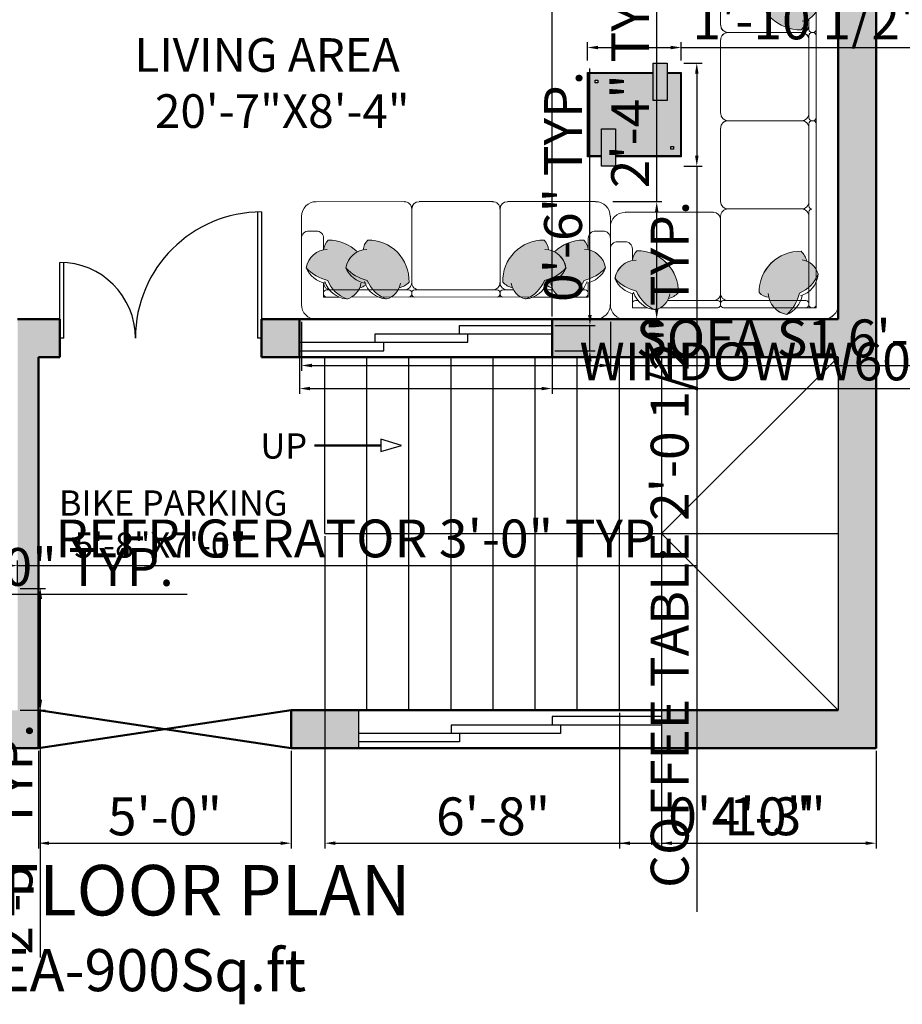
# Model space of a CAD drawing. Units: inches. Extents: x 3274 to 5176, y 1085 to 2172.
# Tile 7 of 16: x 3530 to 3740, y 1614 to 1848. Entities that reach past the tile are written whole.
import ezdxf

# ---------------------------------------------------------------- set-up
doc = ezdxf.new("R2010")
doc.units = ezdxf.units.IN
for name, color, linetype, lineweight in [('A-ANNO-DIMS', 2, 'Continuous', 18), ('A-ANNO-TEXT', 7, 'Continuous', 25), ('A-AREA-IDEN', 3, 'Continuous', 25), ('A-DOOR', 4, 'Continuous', 25), ('A-FLOR-FIXT', 8, 'Continuous', 18), ('A-FLOR-STRS', 7, 'Continuous', 25), ('A-FURN', 8, 'Continuous', 18), ('A-GLAZ', 5, 'Continuous', 25), ('A-WALL', 7, 'Continuous', 50), ('A-WALL-PATT', 8, 'Continuous', 13)]:
    doc.layers.add(name, color=color, linetype=linetype, lineweight=lineweight)
doc.layers.add('MOBIL', color=7, linetype='Continuous')
doc.styles.get("Standard").update_dxf_attribs({"font": 'arial.ttf'})
doc.dimstyles.new('ISO-25', dxfattribs={"dimtxt": 9, "dimasz": 2.5, "dimexe": 1.25, "dimexo": 0.625, "dimtad": 1, "dimdec": 1, "dimlunit": 3, "dimtxsty": 'Standard', "dimcen": 2.5, "dimclrd": 4, "dimclre": 4, "dimclrt": 1, "dimadec": 0, "dimazin": 0, "dimtfac": 1, "dimtdec": 1, "dimtmove": 0, "dimatfit": 3, "dimfxl": 1, "dimarcsym": 0})

# ---------------------------------------------------------------- blocks, each defined once
blk = doc.blocks.new('3')
for p, q in [((47, 30), (47, 0)), ((48, 30), (48, 0)), ((0, 0), (0, 18)), ((1, 0), (1, 18)), ((1, 0), (0, 0)), ((48, 0), (47, 0))]:
    blk.add_line(p, q)
for centre, radius, start, end in [((48, 0), 30, 90, 180), ((0, 0), 18, 0, 90)]:
    blk.add_arc(centre, radius, start, end)
blk = doc.blocks.new('SOFA 1')
at = {"transparency": 33554687}
h = blk.add_hatch(color=256, dxfattribs=at)
h.dxf.hatch_style = 1
h.paths.add_polyline_path([(3723.52, 1308.63, 0.147724), (3717.76, 1305.24, 0.310469), (3722.42, 1300.4), (3722.42, 1300.25, 0.156703), (3723.62, 1297.8, 0.425821), (3734.69, 1309.08, 0.121928), (3732.05, 1310.63, 0.233216), (3728.6, 1313.59, 0.213835)])
h = blk.add_hatch(color=256, dxfattribs=at)
h.dxf.hatch_style = 1
h.paths.add_polyline_path([(3769.65, 1307.6, 0.084911), (3767.15, 1309.12, 0.046133), (3766.46, 1311.13), (3759.18, 1311.13, 0.039409), (3758.92, 1310.24, 0.165523), (3756.31, 1309.02, 0.42585), (3767.59, 1297.95, 0.121928), (3769.15, 1300.58, 0.027403), (3769.65, 1300.83)])
h.paths.add_polyline_path([(3765.34, 1313.08), (3760.4, 1313.08, 0.097704), (3759.18, 1311.13), (3766.46, 1311.13, 0.04873)])
h.paths.add_polyline_path([(3763.76, 1314.88, 0.16488), (3760.4, 1313.08), (3765.34, 1313.08, 0.051917)])
h.paths.add_polyline_path([(3771.6, 1305.17, 0.090388), (3769.65, 1307.6), (3769.65, 1300.83, 0.136035), (3771.6, 1302.77)])
h = blk.add_hatch(color=256, dxfattribs=at)
h.dxf.hatch_style = 1
h.paths.add_polyline_path([(3769.16, 1235.96, 0.122267), (3767.6, 1238.61, 0.425972), (3756.32, 1227.54, 0.165563), (3758.93, 1226.32, 0.309481), (3763.76, 1221.69, 0.002677), (3763.83, 1221.72, 0.146094), (3767.16, 1227.43, 0.212433), (3772.1, 1232.48, 0.235342)])
h = blk.add_hatch(color=256, dxfattribs=at)
h.dxf.hatch_style = 1
h.paths.add_polyline_path([(3769.16, 1225.36, 0.122267), (3767.6, 1228.01, 0.425972), (3756.32, 1216.94, 0.165563), (3758.93, 1215.72, 0.309481), (3763.76, 1211.09, 0.002677), (3763.83, 1211.12, 0.146094), (3767.16, 1216.83, 0.212433), (3772.1, 1221.88, 0.235342)])
for p, q in [((3720.45, 1316.13), (3773.58, 1316.13)), ((3777.51, 1312.19), (3777.51, 1213.72))]:
    blk.add_line(p, q, dxfattribs=at)
for points in [[(3717.76, 1305.24, -0.147724), (3723.52, 1308.63, -0.213355), (3728.59, 1313.59, 0.213355), (3723.52, 1308.63, 0.147724), (3717.76, 1305.24, -0.249545), (3722.86, 1309.34, 0.249545), (3717.75, 1305.25, 0.356779), (3723.4, 1300.28, -0.356779), (3717.76, 1305.24)], [(3728.58, 1313.6, -0.306333), (3732.42, 1309.31, 0.306333), (3728.58, 1313.6, 0.306674), (3722.72, 1308.89, -0.306674), (3728.58, 1313.6)], [(3763.76, 1314.88, -0.147724), (3767.15, 1309.12, -0.213355), (3772.1, 1304.05, 0.213355), (3767.15, 1309.12, 0.147724), (3763.76, 1314.88, -0.249545), (3767.86, 1309.77, 0.249545), (3763.77, 1314.89, 0.356779), (3758.8, 1309.23, -0.356779), (3763.76, 1314.88)], [(3734.69, 1309.08, -0.425972), (3723.62, 1297.8, -0.165552), (3722.4, 1300.4, 0.165552), (3723.62, 1297.79, 0.425972), (3734.69, 1309.07, 0.121514), (3732.07, 1310.63, -0.121514), (3734.69, 1309.08)], [(3767.6, 1297.95, -0.425972), (3756.31, 1309.01, -0.165552), (3758.92, 1310.24, 0.165552), (3756.31, 1309.02, 0.425972), (3767.59, 1297.95, 0.121514), (3769.14, 1300.57, -0.121514), (3767.6, 1297.95)], [(3772.11, 1304.06, -0.306333), (3767.83, 1300.22, 0.306333), (3772.11, 1304.06, 0.306674), (3767.4, 1309.91, -0.306674), (3772.11, 1304.06)], [(3770.44, 1286.63, -0.414214), (3769.66, 1287.4, 0.414214), (3770.44, 1286.63, 0.414214), (3769.66, 1285.83, -0.414214), (3770.44, 1286.63)], [(3748.01, 1262.99, -0.414214), (3746.05, 1264.95, 0.414214), (3748.01, 1262.97, 0.414213), (3746.05, 1261.01, -0.414213), (3748.01, 1262.99)], [(3770.44, 1262.99, -0.414214), (3769.66, 1263.77, 0.414214), (3770.44, 1262.99, 0.414214), (3769.66, 1262.19, -0.414214), (3770.44, 1262.99)], [(3770.83, 1262.97, -0.414214), (3771.61, 1262.19, 0.414214), (3770.83, 1262.99, 0.414214), (3771.61, 1263.77, -0.414214), (3770.83, 1262.97)], [(3748.01, 1239.35, -0.414214), (3746.05, 1241.31, 0.414214), (3748.01, 1239.33, 0.414213), (3746.05, 1237.37, -0.414213), (3748.01, 1239.35)], [(3767.7, 1239.33, -0.414214), (3769.66, 1237.37, 0.414214), (3767.7, 1239.35, 0.414214), (3769.66, 1241.31, -0.414214), (3767.7, 1239.33)], [(3770.44, 1239.35, -0.414214), (3769.66, 1240.13, 0.414214), (3770.44, 1239.33, 0.414214), (3769.66, 1238.55, -0.414214), (3770.44, 1239.35)], [(3770.83, 1239.33, -0.414214), (3771.61, 1238.55, 0.414214), (3770.83, 1239.35, 0.414214), (3771.61, 1240.13, -0.414214), (3770.83, 1239.33)], [(3756.32, 1227.54, -0.425972), (3767.6, 1238.61, -0.121514), (3769.16, 1235.98, 0.121514), (3767.6, 1238.61, 0.425972), (3756.32, 1227.54, 0.165552), (3758.93, 1226.32, -0.165552), (3756.32, 1227.54)], [(3772.1, 1232.5, -0.306674), (3767.41, 1226.64, 0.306674), (3772.1, 1232.5, 0.306333), (3767.84, 1236.34, -0.306333), (3772.1, 1232.5)], [(3763.78, 1221.67, 0.249545), (3767.87, 1226.78, -0.249545), (3763.76, 1221.69, -0.356779), (3758.81, 1227.32, 0.356779), (3763.77, 1221.68, 0.147724), (3767.16, 1227.43, 0.213355), (3772.11, 1232.51, -0.213355), (3767.16, 1227.43, -0.147724), (3763.78, 1221.67)], [(3756.32, 1216.94, -0.200233), (3759.49, 1224.76, 0.200233), (3756.32, 1216.94, 0.165552), (3758.93, 1215.72, -0.165552), (3756.32, 1216.94)], [(3772.1, 1221.9, -0.306674), (3767.41, 1216.04, 0.306674), (3772.1, 1221.9, -0.213355), (3767.16, 1216.83, -0.147724), (3763.77, 1211.08, 0.147724), (3767.15, 1216.83, 0.213355), (3772.1, 1221.9)], [(3763.76, 1211.09, -0.356779), (3758.81, 1216.72, 0.356779), (3763.76, 1211.09, 0.249545), (3767.87, 1216.18, -0.249545), (3763.76, 1211.09)]]:
    blk.add_lwpolyline(points, format="xyb", dxfattribs=at)
for points in [[(3716.51, 1312.2), (3716.51, 1291.44)], [(3722.42, 1313.08), (3722.42, 1309.23), (3722.42, 1313.08), (3726.57, 1313.08)], [(3723.21, 1311.13), (3723.93, 1311.13)], [(3729.85, 1313.08), (3745.25, 1313.08)], [(3731.82, 1311.13), (3745.25, 1311.13)], [(3746.01, 1312.3), (3746.01, 1288.55)], [(3746.01, 1310.97), (3746.01, 1311.36)], [(3768.11, 1313.08), (3746.78, 1313.08)], [(3768.87, 1311.13), (3746.78, 1311.13)], [(3771.6, 1313.08), (3767.75, 1313.08), (3771.6, 1313.08), (3771.6, 1308.93)], [(3769.66, 1287.39), (3769.65, 1312.3)], [(3771.6, 1313.08), (3771.61, 1233.74)], [(3746.01, 1288.54), (3746.01, 1308.23)], [(3769.65, 1309.43), (3769.65, 1308.71)], [(3722.42, 1300.39), (3722.42, 1297.33)], [(3720.45, 1295.38), (3718.48, 1295.38)], [(3720.45, 1287.5), (3744.09, 1287.5)], [(3746.02, 1284.63), (3746.02, 1264.94)], [(3747.99, 1286.6), (3767.69, 1286.6)], [(3769.66, 1263.75), (3769.66, 1285.81)], [(3769.66, 1277.18), (3769.66, 1263.75)], [(3746.02, 1260.99), (3746.02, 1241.3)], [(3747.99, 1262.97), (3767.69, 1262.97)], [(3769.66, 1240.12), (3769.66, 1262.18)], [(3770.43, 1262.97), (3770.82, 1262.97)], [(3746.02, 1237.36), (3746.02, 1213.74)], [(3747.99, 1239.33), (3767.69, 1239.33)], [(3769.66, 1235.71), (3769.66, 1238.54)], [(3770.43, 1239.33), (3770.82, 1239.33)], [(3771.61, 1223.14), (3771.61, 1230.47)], [(3769.66, 1225.11), (3769.66, 1227.82)], [(3767.76, 1215.72), (3771.61, 1215.72), (3771.61, 1219.84), (3771.61, 1215.72)], [(3769.66, 1216.5), (3769.66, 1217.22)], [(3753.91, 1211.77), (3753.91, 1213.74)], [(3755.86, 1215.72), (3758.92, 1215.72)], [(3749.97, 1209.8), (3773.58, 1209.8)]]:
    blk.add_lwpolyline(points, close=True, dxfattribs=at)
for points in [[(3722.42, 1311.91, 0.414214), (3723.2, 1311.13, -0.414214)], [(3770.43, 1313.08, 0.414214), (3769.65, 1312.3, -0.414214)], [(3771.6, 1312.3, 0.414214), (3770.82, 1313.08, -0.414214)], [(3716.51, 1297.34, 0.414214), (3718.47, 1295.38, -0.414214)], [(3720.44, 1295.38, 0.414214), (3722.4, 1297.34, -0.414214)], [(3716.51, 1291.45, 0.414212), (3720.44, 1287.52, -0.414212)], [(3746.03, 1288.56, 0.414214), (3747.99, 1286.6, 0.414213), (3746.03, 1284.64, -0.414213), (3747.99, 1286.6, -0.414214)], [(3769.66, 1284.64, 0.414214), (3767.7, 1286.6, 0.414214), (3769.66, 1288.56, -0.414214), (3767.7, 1286.6, -0.414214)], [(3769.66, 1261.01, 0.414214), (3767.7, 1262.97, 0.414214), (3769.66, 1264.93, -0.414214), (3767.7, 1262.97, -0.414214)], [(3769.16, 1225.36, 0.071861), (3768.39, 1227.01, -0.071861)], [(3772.13, 1221.9, 0.306333), (3767.84, 1225.74, -0.306333)], [(3769.66, 1216.52, 0.414214), (3770.44, 1215.74, -0.414214)], [(3770.83, 1215.74, 0.414214), (3771.61, 1216.52, -0.414214)], [(3746.05, 1213.76, 0.414212), (3749.98, 1209.82, -0.414212)], [(3755.87, 1215.72, 0.414214), (3753.91, 1213.76, -0.414214)], [(3755.87, 1209.8, -0.414214), (3753.91, 1211.76, 0.414214)]]:
    blk.add_lwpolyline(points, format="xyb", close=True, dxfattribs=at)
for centre, radius, start, end in [((3720.44, 1312.2), 3.93, 90.0002, 179.9998), ((3720.44, 1312.19), 3.94, 89.9158, 179.9154), ((3773.58, 1312.2), 3.93, 0.0002, 89.9998), ((3773.57, 1312.19), 3.94, 359.9158, 89.9154), ((3744.09, 1309.21), 1.92, 358.766, 90.5111), ((3745.22, 1312.29), 0.789, 0.8425, 90.8425), ((3745.24, 1311.91), 0.777, 270, 0), ((3745.24, 1311.91), 0.777, 270, 0), ((3746.8, 1312.29), 0.789, 89.1575, 179.1575), ((3746.79, 1311.91), 0.777, 180, 270), ((3746.79, 1311.91), 0.777, 180, 270), ((3747.93, 1309.21), 1.92, 89.4889, 181.234), ((3768.87, 1312.3), 0.777, 360, 90), ((3768.87, 1311.91), 0.777, 270, 0), ((3744.08, 1289.48), 1.96, 270, 360), ((3744.08, 1289.48), 1.96, 270, 360), ((3773.58, 1213.73), 3.93, 270.0002, 359.9998), ((3773.59, 1213.73), 3.93, 269.9156, 359.9152)]:
    blk.add_arc(centre, radius, start, end, dxfattribs=at)
blk = doc.blocks.new('Mesa de centro Cantria feeling')
at = {"layer": 'MOBIL', "ltscale": 0.2}
h = blk.add_hatch(color=256, dxfattribs=at)
h.set_gradient(color1=(74, 55, 38), color2=(104, 77, 54), one_color=1, tint=0.31, name='CYLINDER')
h.paths.add_polyline_path([(-0.85, -0.3), (-0.7, -0.3), (-0.7, 0.1), (-0.85, 0.1)])
h = blk.add_hatch(color=256, dxfattribs=at)
h.set_gradient(color1=(221, 221, 223), one_color=1, tint=1)
h.paths.add_polyline_path([(-0.15, -0.6), (-0.15, -0.89), (-0.01, -0.89), (-0.01, -0.01), (-0.7, -0.01), (-0.7, -0.3), (-0.85, -0.3), (-0.85, -0.01), (-0.99, -0.01), (-0.99, -0.89), (-0.3, -0.89), (-0.3, -0.6)])
h.paths.add_polyline_path([(-0.112, -0.112), (-0.112, -0.082), (-0.082, -0.082), (-0.082, -0.112)], flags=16)
h.paths.add_polyline_path([(-0.888, -0.788), (-0.888, -0.818), (-0.918, -0.818), (-0.918, -0.788)], flags=16)
h = blk.add_hatch(color=256, dxfattribs=at)
h.set_gradient(color1=(74, 55, 38), color2=(104, 77, 54), one_color=1, tint=0.31, name='CYLINDER')
h.paths.add_polyline_path([(-0.15, -0.6), (-0.3, -0.6), (-0.3, -1), (-0.15, -1)])
for points in [[(-0.85, 0), (-1, 0), (-1, -0.9), (-0.3, -0.9)], [(-0.15, -0.9), (0, -0.9), (0, 0), (-0.7, 0)], [(-0.85, -0.01), (-0.99, -0.01), (-0.99, -0.89), (-0.3, -0.89)], [(-0.15, -0.89), (-0.01, -0.89), (-0.01, -0.01), (-0.7, -0.01)]]:
    blk.add_lwpolyline(points, dxfattribs=at)
for points in [[(-0.85, -0.3), (-0.7, -0.3), (-0.7, 0.1), (-0.85, 0.1)], [(-0.082, -0.082), (-0.112, -0.082), (-0.112, -0.112), (-0.082, -0.112)], [(-0.15, -0.6), (-0.3, -0.6), (-0.3, -1), (-0.15, -1)], [(-0.918, -0.818), (-0.888, -0.818), (-0.888, -0.788), (-0.918, -0.788)]]:
    blk.add_lwpolyline(points, close=True, dxfattribs=at)
blk = doc.blocks.new('S1')
at = {"transparency": 33554687}
h = blk.add_hatch(color=256, dxfattribs=at)
h.dxf.hatch_style = 1
h.paths.add_polyline_path([(3706.22, 1117.89, 0.122267), (3708.57, 1119.27, 0.425972), (3698.75, 1129.29, 0.165563), (3697.66, 1126.97, 0.309481), (3693.55, 1122.68, 0.002677), (3693.58, 1122.62, 0.146094), (3698.65, 1119.67, 0.212433), (3703.13, 1115.28, 0.235342)])
h = blk.add_hatch(color=256, dxfattribs=at)
h.dxf.hatch_style = 1
h.paths.add_polyline_path([(3715.63, 1117.89, 0.122267), (3717.98, 1119.27, 0.425972), (3708.16, 1129.29, 0.165563), (3707.07, 1126.97, 0.309481), (3702.96, 1122.68, 0.002677), (3702.99, 1122.62, 0.146094), (3708.06, 1119.67, 0.212433), (3712.54, 1115.28, 0.235342)])
h = blk.add_hatch(color=256, dxfattribs=at)
h.dxf.hatch_style = 1
h.paths.add_polyline_path([(3742.59, 1117.89, -0.122267), (3740.24, 1119.27, -0.425972), (3750.07, 1129.29, -0.165563), (3751.15, 1126.97, -0.309481), (3755.26, 1122.68, -0.002677), (3755.24, 1122.62, -0.146094), (3750.16, 1119.67, -0.212433), (3745.68, 1115.28, -0.235342)])
h = blk.add_hatch(color=256, dxfattribs=at)
h.dxf.hatch_style = 1
h.paths.add_polyline_path([(3752, 1117.89, -0.122267), (3749.65, 1119.27, -0.425972), (3759.48, 1129.29, -0.165563), (3760.56, 1126.97, -0.309481), (3764.67, 1122.68, -0.002677), (3764.65, 1122.62, -0.146094), (3759.57, 1119.67, -0.212433), (3755.09, 1115.28, -0.235342)])
for p, q in [((3747.47, 1115.72), (3704.36, 1115.76)), ((3695.9, 1110.48), (3762.33, 1110.48))]:
    blk.add_line(p, q)
for points in [[(3695.92, 1138.41, 0.414212), (3692.43, 1134.92, -0.414212)], [(3762.3, 1138.41, -0.414212), (3765.79, 1134.92, 0.414212)], [(3692.41, 1129.69, -0.414214), (3694.15, 1131.43, 0.414214)], [(3697.66, 1129.69, 0.414214), (3695.92, 1131.43, -0.414214)], [(3760.56, 1129.69, -0.414214), (3762.3, 1131.43, 0.414214)], [(3765.81, 1129.69, 0.414214), (3764.07, 1131.43, -0.414214)], [(3703.15, 1115.26, 0.306333), (3706.55, 1119.07, -0.306333)], [(3720.36, 1117.45, -0.414214), (3718.62, 1119.19, -0.414214), (3716.88, 1117.45, 0.414214), (3718.62, 1119.19, 0.414214)], [(3755.08, 1115.26, -0.306333), (3751.67, 1119.07, 0.306333)], [(3698.37, 1117.45, 0.414214), (3697.68, 1116.76, -0.414214)], [(3706.22, 1117.89, 0.071861), (3707.68, 1118.58, -0.071861)], [(3752, 1117.89, -0.071861), (3750.54, 1118.58, 0.071861)], [(3759.85, 1117.45, -0.414214), (3760.54, 1116.76, 0.414214)], [(3697.68, 1116.41, 0.414214), (3698.37, 1115.72, -0.414214)], [(3760.54, 1116.41, -0.414214), (3759.85, 1115.72, 0.414214)]]:
    blk.add_lwpolyline(points, format="xyb", close=True, dxfattribs=at)
for points in [[(3695.92, 1138.41), (3716.87, 1138.43)], [(3720.37, 1138.43), (3737.85, 1138.43)], [(3741.35, 1138.43), (3762.31, 1138.43)], [(3718.62, 1136.68), (3718.62, 1119.2)], [(3739.6, 1136.68), (3739.6, 1119.2)], [(3692.41, 1134.93), (3692.41, 1113.97)], [(3692.41, 1134.81), (3692.41, 1113.85)], [(3765.81, 1134.93), (3765.81, 1113.97)], [(3694.16, 1131.43), (3695.91, 1131.43)], [(3764.06, 1131.43), (3762.31, 1131.43)], [(3697.66, 1129.7), (3697.66, 1126.98)], [(3760.56, 1129.7), (3760.56, 1126.98)], [(3697.66, 1119.14), (3697.66, 1115.72), (3701.32, 1115.72), (3697.66, 1115.72)], [(3760.56, 1119.14), (3760.56, 1115.72), (3756.9, 1115.72), (3760.56, 1115.72)], [(3717.92, 1117.45), (3698.34, 1117.45)], [(3698.35, 1117.46), (3698.99, 1117.46)], [(3698.36, 1117.45), (3699, 1117.45)], [(3706, 1117.45), (3717.92, 1117.45)], [(3718.62, 1116.77), (3718.62, 1116.42)], [(3738.9, 1117.45), (3719.32, 1117.45)], [(3739.6, 1116.77), (3739.6, 1116.42)], [(3742.81, 1117.45), (3740.3, 1117.45)], [(3752.22, 1117.45), (3749.81, 1117.45)], [(3759.86, 1117.45), (3759.22, 1117.45)], [(3753.97, 1115.72), (3747.47, 1115.72)]]:
    blk.add_lwpolyline(points, close=True, dxfattribs=at)
for points in [[(3718.6, 1136.67, 0.414214), (3716.86, 1138.41, -0.414214), (3718.62, 1136.67, -0.414213), (3720.36, 1138.41, 0.414213), (3718.6, 1136.67)], [(3739.58, 1136.67, 0.414214), (3737.84, 1138.41, -0.414214), (3739.6, 1136.67, -0.414213), (3741.34, 1138.41, 0.414213), (3739.58, 1136.67)], [(3698.75, 1129.29, -0.200233), (3705.69, 1126.47, 0.200233), (3698.75, 1129.29, 0.165552), (3697.66, 1126.97, -0.165552), (3698.75, 1129.29)], [(3708.16, 1129.29, -0.425972), (3717.98, 1119.27, -0.121514), (3715.65, 1117.89, 0.121514), (3717.98, 1119.27, 0.425972), (3708.16, 1129.29, 0.165552), (3707.07, 1126.97, -0.165552), (3708.16, 1129.29)], [(3750.07, 1129.29, 0.425972), (3740.24, 1119.27, 0.121514), (3742.57, 1117.89, -0.121514), (3740.24, 1119.27, -0.425972), (3750.07, 1129.29, -0.165552), (3751.15, 1126.97, 0.165552), (3750.07, 1129.29)], [(3759.48, 1129.29, 0.200233), (3752.53, 1126.47, -0.200233), (3759.48, 1129.29, -0.165552), (3760.56, 1126.97, 0.165552), (3759.48, 1129.29)], [(3693.55, 1122.68, -0.356779), (3698.55, 1127.08, 0.356779), (3693.55, 1122.68, 0.249545), (3698.07, 1119.04, -0.249545), (3693.55, 1122.68)], [(3702.94, 1122.67, 0.249545), (3707.48, 1119.04, -0.249545), (3702.96, 1122.68, -0.356779), (3707.96, 1127.08, 0.356779), (3702.95, 1122.67, 0.147724), (3708.06, 1119.67, 0.213355), (3712.56, 1115.27, -0.213355), (3708.06, 1119.67, -0.147724), (3702.94, 1122.67)], [(3755.28, 1122.67, -0.249545), (3750.74, 1119.04, 0.249545), (3755.26, 1122.68, 0.356779), (3750.26, 1127.08, -0.356779), (3755.27, 1122.67, -0.147724), (3750.16, 1119.67, -0.213355), (3745.66, 1115.27, 0.213355), (3750.16, 1119.67, 0.147724), (3755.28, 1122.67)], [(3764.67, 1122.68, 0.356779), (3759.67, 1127.08, -0.356779), (3764.67, 1122.68, -0.249545), (3760.15, 1119.04, 0.249545), (3764.67, 1122.68)], [(3703.15, 1115.28, -0.306674), (3697.95, 1119.44, 0.306674), (3703.15, 1115.28, -0.213355), (3698.65, 1119.67, -0.147724), (3693.54, 1122.67, 0.147724), (3698.65, 1119.67, 0.213355), (3703.15, 1115.28)], [(3755.07, 1115.28, 0.306674), (3760.27, 1119.44, -0.306674), (3755.07, 1115.28, 0.213355), (3759.57, 1119.67, 0.147724), (3764.68, 1122.67, -0.147724), (3759.57, 1119.67, -0.213355), (3755.07, 1115.28)], [(3712.56, 1115.28, -0.306674), (3707.36, 1119.44, 0.306674), (3712.56, 1115.28, 0.306333), (3715.96, 1119.07, -0.306333), (3712.56, 1115.28)], [(3739.6, 1119.19, 0.414214), (3741.34, 1117.45, -0.414214), (3739.58, 1119.19, -0.414214), (3737.84, 1117.45, 0.414214), (3739.6, 1119.19)], [(3745.66, 1115.28, 0.306674), (3750.86, 1119.44, -0.306674), (3745.66, 1115.28, -0.306333), (3742.26, 1119.07, 0.306333), (3745.66, 1115.28)], [(3718.6, 1116.76, 0.414214), (3717.91, 1117.45, -0.414214), (3718.6, 1116.76, -0.414214), (3719.31, 1117.45, 0.414214), (3718.6, 1116.76)], [(3739.58, 1116.76, 0.414214), (3738.89, 1117.45, -0.414214), (3739.6, 1116.76, -0.414214), (3740.29, 1117.45, 0.414214), (3739.58, 1116.76)], [(3718.62, 1116.41, 0.414214), (3719.31, 1115.72, -0.414214), (3718.6, 1116.41, -0.414214), (3717.91, 1115.72, 0.414214), (3718.62, 1116.41)], [(3739.6, 1116.41, 0.414214), (3740.29, 1115.72, -0.414214), (3739.58, 1116.41, -0.414214), (3738.89, 1115.72, 0.414214), (3739.6, 1116.41)]]:
    blk.add_lwpolyline(points, format="xyb", dxfattribs=at)
for centre, radius, start, end in [((3699.38, 1119.19), 1.74, 180, 270), ((3699.38, 1119.19), 1.74, 180, 270), ((3695.9, 1113.97), 3.5, 180.0846, 270.0842), ((3762.32, 1113.97), 3.49, 270.0002, 359.9998), ((3762.33, 1113.96), 3.48, 270.0848, 0.0844)]:
    blk.add_arc(centre, radius, start, end, dxfattribs=at)
blk = doc.blocks.new('WIN-60')
for p, q in [((4618.19, 1273.85), (4640.19, 1273.85)), ((4618.19, 1271.85), (4618.19, 1273.85)), ((4598.19, 1271.85), (4640.19, 1271.85)), ((4598.19, 1269.85), (4598.19, 1271.85)), ((4620.19, 1269.85), (4620.19, 1271.85)), ((4580.19, 1269.85), (4620.19, 1269.85)), ((4600.19, 1267.85), (4600.19, 1269.85)), ((4580.19, 1267.85), (4600.19, 1267.85))]:
    blk.add_line(p, q)
blk = doc.blocks.new('WIN-72')
for p, q in [((4462.19, 1180.85), (4436.19, 1180.85)), ((4436.19, 1180.85), (4436.19, 1178.85)), ((4462.19, 1178.85), (4412.19, 1178.85)), ((4412.19, 1178.85), (4412.19, 1176.85)), ((4438.19, 1178.85), (4438.19, 1176.85)), ((4438.19, 1176.85), (4390.19, 1176.85)), ((4414.19, 1176.85), (4414.19, 1174.85)), ((4414.19, 1174.85), (4390.19, 1174.85))]:
    blk.add_line(p, q)
blk = doc.blocks.new('*D128')
at = {"layer": 'A-ANNO-DIMS', "color": 4, "lineweight": -2, "transparency": 16777216}
for p, q in [((3596.3, 1768.36), (3596.3, 1758.73)), ((3656.3, 1768.36), (3656.3, 1758.73)), ((3598.8, 1759.98), (3653.8, 1759.98)), ((3656.3, 1759.98), (3803.28, 1759.98))]:
    blk.add_line(p, q, dxfattribs=at)
at = {"layer": 'A-ANNO-DIMS', "color": 4, "transparency": 16777216}
for points in [[(3598.8, 1760.4), (3598.8, 1759.57), (3596.3, 1759.98)], [(3653.8, 1760.4), (3653.8, 1759.57), (3656.3, 1759.98)]]:
    blk.add_solid(points, dxfattribs=at)
at = {"layer": 'Defpoints', "color": 0, "transparency": 16777216}
for p in [(3596.3, 1768.98), (3656.3, 1768.98), (3656.3, 1759.98)]:
    blk.add_point(p, dxfattribs=at)
at = {"layer": 'A-ANNO-DIMS', "color": 1, "transparency": 16777216, "insert": (3731.04, 1765.26), "char_height": 9, "attachment_point": 5}
blk.add_mtext('WINDOW W60 5\'-0" TYP.', dxfattribs=at)
blk = doc.blocks.new('*D129')
at = {"layer": 'A-ANNO-DIMS', "color": 4, "lineweight": -2, "transparency": 16777216}
for p, q in [((3665.3, 1777.48), (3665.3, 1836.09)), ((3656.93, 1774.98), (3666.55, 1774.98)), ((3665.3, 1768.98), (3665.3, 1774.98)), ((3656.93, 1768.98), (3666.55, 1768.98)), ((3665.3, 1766.48), (3665.3, 1763.98))]:
    blk.add_line(p, q, dxfattribs=at)
at = {"layer": 'A-ANNO-DIMS', "color": 4, "transparency": 16777216}
for points in [[(3664.88, 1777.48), (3665.72, 1777.48), (3665.3, 1774.98)], [(3664.88, 1766.48), (3665.72, 1766.48), (3665.3, 1768.98)]]:
    blk.add_solid(points, dxfattribs=at)
at = {"layer": 'Defpoints', "color": 0, "transparency": 16777216}
for p in [(3656.3, 1774.98), (3665.3, 1774.98), (3656.3, 1768.98)]:
    blk.add_point(p, dxfattribs=at)
at = {"layer": 'A-ANNO-DIMS', "color": 1, "transparency": 16777216, "insert": (3660.08, 1808.04), "char_height": 9, "attachment_point": 5, "rotation": 90}
blk.add_mtext('0\'-6" TYP.', dxfattribs=at)
blk = doc.blocks.new('*D134')
at = {"layer": 'A-ANNO-DIMS', "color": 4, "lineweight": -2, "transparency": 16777216}
for p, q in [((3428.94, 1706.35), (3428.94, 1712.37)), ((3464.94, 1706.35), (3464.94, 1712.37)), ((3431.44, 1711.12), (3462.44, 1711.12)), ((3464.94, 1711.12), (3569.61, 1711.12))]:
    blk.add_line(p, q, dxfattribs=at)
at = {"layer": 'A-ANNO-DIMS', "color": 4, "transparency": 16777216}
for points in [[(3431.44, 1711.54), (3431.44, 1710.7), (3428.94, 1711.12)], [(3462.44, 1711.54), (3462.44, 1710.7), (3464.94, 1711.12)]]:
    blk.add_solid(points, dxfattribs=at)
at = {"layer": 'Defpoints', "color": 0, "transparency": 16777216}
for p in [(3464.94, 1711.12), (3428.94, 1705.72), (3464.94, 1705.72)]:
    blk.add_point(p, dxfattribs=at)
at = {"layer": 'A-ANNO-DIMS', "color": 1, "transparency": 16777216, "insert": (3518.52, 1716.4), "char_height": 9, "attachment_point": 5}
blk.add_mtext('STOVE 3\'-0" TYP.', dxfattribs=at)
blk = doc.blocks.new('*D138')
at = {"layer": 'A-ANNO-DIMS', "color": 4, "lineweight": -2, "transparency": 16777216}
for p, q in [((3687.65, 1837.38), (3691.95, 1837.38)), ((3690.7, 1834.88), (3690.7, 1815.34)), ((3687.65, 1812.84), (3691.95, 1812.84)), ((3690.7, 1812.84), (3690.7, 1635.55))]:
    blk.add_line(p, q, dxfattribs=at)
at = {"layer": 'A-ANNO-DIMS', "color": 4, "transparency": 16777216}
for points in [[(3690.29, 1834.88), (3691.12, 1834.88), (3690.7, 1837.38)], [(3690.29, 1815.34), (3691.12, 1815.34), (3690.7, 1812.84)]]:
    blk.add_solid(points, dxfattribs=at)
at = {"layer": 'Defpoints', "color": 0, "transparency": 16777216}
for p in [(3687.02, 1837.38), (3687.02, 1812.84), (3690.7, 1812.84)]:
    blk.add_point(p, dxfattribs=at)
at = {"layer": 'A-ANNO-DIMS', "color": 1, "transparency": 16777216, "insert": (3685.42, 1722.94), "char_height": 9, "attachment_point": 5, "rotation": 90}
blk.add_mtext('COFFEE TABLE 2\'-0 1/2" TYP.', dxfattribs=at)
blk = doc.blocks.new('*D139')
at = {"layer": 'A-ANNO-DIMS', "color": 4, "lineweight": -2, "transparency": 16777216}
for p, q in [((3664.71, 1838.01), (3664.71, 1842.31)), ((3667.21, 1841.06), (3684.52, 1841.06)), ((3687.02, 1838.01), (3687.02, 1842.31)), ((3687.02, 1841.06), (3772.75, 1841.06))]:
    blk.add_line(p, q, dxfattribs=at)
at = {"layer": 'A-ANNO-DIMS', "color": 4, "transparency": 16777216}
for points in [[(3667.21, 1841.48), (3667.21, 1840.65), (3664.71, 1841.06)], [(3684.52, 1841.48), (3684.52, 1840.65), (3687.02, 1841.06)]]:
    blk.add_solid(points, dxfattribs=at)
at = {"layer": 'Defpoints', "color": 0, "transparency": 16777216}
for p in [(3687.02, 1841.06), (3664.71, 1837.38), (3687.02, 1837.38)]:
    blk.add_point(p, dxfattribs=at)
at = {"layer": 'A-ANNO-DIMS', "color": 1, "transparency": 16777216, "insert": (3731.13, 1846.34), "char_height": 9, "attachment_point": 5}
blk.add_mtext('1\'-10 1/2" TYP.', dxfattribs=at)
blk = doc.blocks.new('*D140')
at = {"layer": 'A-ANNO-DIMS', "color": 4, "lineweight": -2, "transparency": 16777216}
for p, q in [((3596.75, 1775.85), (3596.75, 1764.21)), ((3670.16, 1775.85), (3670.16, 1764.21)), ((3599.25, 1765.46), (3667.66, 1765.46)), ((3670.16, 1765.46), (3806.3, 1765.46))]:
    blk.add_line(p, q, dxfattribs=at)
at = {"layer": 'A-ANNO-DIMS', "color": 4, "transparency": 16777216}
for points in [[(3599.25, 1765.88), (3599.25, 1765.04), (3596.75, 1765.46)], [(3667.66, 1765.88), (3667.66, 1765.04), (3670.16, 1765.46)]]:
    blk.add_solid(points, dxfattribs=at)
at = {"layer": 'Defpoints', "color": 0, "transparency": 16777216}
for p in [(3596.75, 1776.47), (3670.16, 1776.47), (3670.16, 1765.46)]:
    blk.add_point(p, dxfattribs=at)
at = {"layer": 'A-ANNO-DIMS', "color": 1, "transparency": 16777216, "insert": (3739.48, 1770.74), "char_height": 9, "attachment_point": 5}
blk.add_mtext('SOFA S1 6\'-1 1/2" TYP.', dxfattribs=at)
blk = doc.blocks.new('*D141')
at = {"layer": 'A-ANNO-DIMS', "color": 4, "lineweight": -2, "transparency": 16777216}
for p, q in [((3681.18, 1804.42), (3681.18, 1863.19)), ((3670.79, 1804.42), (3682.43, 1804.42)), ((3681.18, 1778.97), (3681.18, 1801.92)), ((3670.79, 1776.47), (3682.43, 1776.47))]:
    blk.add_line(p, q, dxfattribs=at)
at = {"layer": 'A-ANNO-DIMS', "color": 4, "transparency": 16777216}
for points in [[(3680.76, 1801.92), (3681.59, 1801.92), (3681.18, 1804.42)], [(3680.76, 1778.97), (3681.59, 1778.97), (3681.18, 1776.47)]]:
    blk.add_solid(points, dxfattribs=at)
at = {"layer": 'Defpoints', "color": 0, "transparency": 16777216}
for p in [(3670.16, 1804.42), (3681.18, 1804.42), (3670.16, 1776.47)]:
    blk.add_point(p, dxfattribs=at)
at = {"layer": 'A-ANNO-DIMS', "color": 1, "transparency": 16777216, "insert": (3676.03, 1835.06), "char_height": 9, "attachment_point": 5, "rotation": 90}
blk.add_mtext('2\'-4" TYP.', dxfattribs=at)
blk = doc.blocks.new('*D142')
at = {"layer": 'A-ANNO-DIMS', "color": 4, "lineweight": -2, "transparency": 16777216}
for p, q in [((3493.3, 1713.11), (3493.3, 1719.13)), ((3529.3, 1713.11), (3529.3, 1719.13)), ((3495.8, 1717.88), (3526.8, 1717.88)), ((3529.3, 1717.88), (3690.83, 1717.88))]:
    blk.add_line(p, q, dxfattribs=at)
at = {"layer": 'A-ANNO-DIMS', "color": 4, "transparency": 16777216}
for points in [[(3495.8, 1718.3), (3495.8, 1717.47), (3493.3, 1717.88)], [(3526.8, 1718.3), (3526.8, 1717.47), (3529.3, 1717.88)]]:
    blk.add_solid(points, dxfattribs=at)
at = {"layer": 'Defpoints', "color": 0, "transparency": 16777216}
for p in [(3529.3, 1717.88), (3493.3, 1712.48), (3529.3, 1712.48)]:
    blk.add_point(p, dxfattribs=at)
at = {"layer": 'A-ANNO-DIMS', "color": 1, "transparency": 16777216, "insert": (3611.31, 1723.17), "char_height": 9, "attachment_point": 5}
blk.add_mtext('REFRIGERATOR 3\'-0" TYP.', dxfattribs=at)
blk = doc.blocks.new('*D143')
at = {"layer": 'A-ANNO-DIMS', "color": 4, "lineweight": -2, "transparency": 16777216}
for p, q in [((3529.93, 1712.48), (3535.95, 1712.48)), ((3534.7, 1709.98), (3534.7, 1685.98)), ((3529.93, 1683.48), (3535.95, 1683.48)), ((3534.7, 1683.48), (3534.7, 1624.72))]:
    blk.add_line(p, q, dxfattribs=at)
at = {"layer": 'A-ANNO-DIMS', "color": 4, "transparency": 16777216}
for points in [[(3534.28, 1709.98), (3535.12, 1709.98), (3534.7, 1712.48)], [(3534.28, 1685.98), (3535.12, 1685.98), (3534.7, 1683.48)]]:
    blk.add_solid(points, dxfattribs=at)
at = {"layer": 'Defpoints', "color": 0, "transparency": 16777216}
for p in [(3529.3, 1712.48), (3529.3, 1683.48), (3534.7, 1683.48)]:
    blk.add_point(p, dxfattribs=at)
at = {"layer": 'A-ANNO-DIMS', "color": 1, "transparency": 16777216, "insert": (3529.48, 1652.85), "char_height": 9, "attachment_point": 5, "rotation": 90}
blk.add_mtext('2\'-5" TYP.', dxfattribs=at)
blk = doc.blocks.new('*D168')
at = {"layer": 'A-ANNO-DIMS', "color": 4, "lineweight": -2, "transparency": 16777216}
for p, q in [((3682.3, 1673.86), (3682.3, 1650.63)), ((3733.3, 1673.86), (3733.3, 1650.63)), ((3684.8, 1651.88), (3730.8, 1651.88))]:
    blk.add_line(p, q, dxfattribs=at)
at = {"layer": 'A-ANNO-DIMS', "color": 4, "transparency": 16777216}
for points in [[(3684.8, 1652.3), (3684.8, 1651.47), (3682.3, 1651.88)], [(3730.8, 1652.3), (3730.8, 1651.47), (3733.3, 1651.88)]]:
    blk.add_solid(points, dxfattribs=at)
at = {"layer": 'Defpoints', "color": 0, "transparency": 16777216}
for p in [(3682.3, 1674.48), (3733.3, 1674.48), (3733.3, 1651.88)]:
    blk.add_point(p, dxfattribs=at)
at = {"layer": 'A-ANNO-DIMS', "color": 1, "transparency": 16777216, "insert": (3707.8, 1657.11), "char_height": 9, "attachment_point": 5}
blk.add_mtext('4\'-3"', dxfattribs=at)
blk = doc.blocks.new('*D169')
at = {"layer": 'A-ANNO-DIMS', "color": 4, "lineweight": -2, "transparency": 16777216}
for p, q in [((3534.3, 1673.86), (3534.3, 1650.63)), ((3594.3, 1673.86), (3594.3, 1650.63)), ((3536.8, 1651.88), (3591.8, 1651.88))]:
    blk.add_line(p, q, dxfattribs=at)
at = {"layer": 'A-ANNO-DIMS', "color": 4, "transparency": 16777216}
for points in [[(3536.8, 1652.3), (3536.8, 1651.47), (3534.3, 1651.88)], [(3591.8, 1652.3), (3591.8, 1651.47), (3594.3, 1651.88)]]:
    blk.add_solid(points, dxfattribs=at)
at = {"layer": 'Defpoints', "color": 0, "transparency": 16777216}
for p in [(3534.3, 1674.48), (3594.3, 1674.48), (3594.3, 1651.88)]:
    blk.add_point(p, dxfattribs=at)
at = {"layer": 'A-ANNO-DIMS', "color": 1, "transparency": 16777216, "insert": (3564.3, 1657.1), "char_height": 9, "attachment_point": 5}
blk.add_mtext('5\'-0"', dxfattribs=at)
blk = doc.blocks.new('*D172')
at = {"layer": 'A-ANNO-DIMS', "color": 4, "lineweight": -2, "transparency": 16777216}
for p, q in [((3602.3, 1724.86), (3602.3, 1650.63)), ((3682.3, 1724.86), (3682.3, 1650.63)), ((3604.8, 1651.88), (3679.8, 1651.88))]:
    blk.add_line(p, q, dxfattribs=at)
at = {"layer": 'A-ANNO-DIMS', "color": 4, "transparency": 16777216}
for points in [[(3604.8, 1652.3), (3604.8, 1651.47), (3602.3, 1651.88)], [(3679.8, 1652.3), (3679.8, 1651.47), (3682.3, 1651.88)]]:
    blk.add_solid(points, dxfattribs=at)
at = {"layer": 'Defpoints', "color": 0, "transparency": 16777216}
for p in [(3602.3, 1725.48), (3682.3, 1725.48), (3682.3, 1651.88)]:
    blk.add_point(p, dxfattribs=at)
at = {"layer": 'A-ANNO-DIMS', "color": 1, "transparency": 16777216, "insert": (3642.3, 1657.1), "char_height": 9, "attachment_point": 5}
blk.add_mtext('6\'-8"', dxfattribs=at)
blk = doc.blocks.new('*D173')
at = {"layer": 'A-ANNO-DIMS', "color": 4, "lineweight": -2, "transparency": 16777216}
for p, q in [((3672.3, 1682.86), (3672.3, 1650.63)), ((3682.3, 1682.86), (3682.3, 1650.63)), ((3674.8, 1651.88), (3679.8, 1651.88)), ((3682.3, 1651.88), (3716.97, 1651.88))]:
    blk.add_line(p, q, dxfattribs=at)
at = {"layer": 'A-ANNO-DIMS', "color": 4, "transparency": 16777216}
for points in [[(3674.8, 1652.3), (3674.8, 1651.47), (3672.3, 1651.88)], [(3679.8, 1652.3), (3679.8, 1651.47), (3682.3, 1651.88)]]:
    blk.add_solid(points, dxfattribs=at)
at = {"layer": 'Defpoints', "color": 0, "transparency": 16777216}
for p in [(3672.3, 1683.48), (3682.3, 1683.48), (3682.3, 1651.88)]:
    blk.add_point(p, dxfattribs=at)
at = {"layer": 'A-ANNO-DIMS', "color": 1, "transparency": 16777216, "insert": (3700.88, 1657.1), "char_height": 9, "attachment_point": 5}
blk.add_mtext('0\'-10"', dxfattribs=at)
blk = doc.blocks.new('*D174')
at = {"layer": 'A-ANNO-DIMS', "color": 4, "lineweight": -2, "transparency": 16777216}
for p, q in [((3656.3, 1777.11), (3656.3, 2058.33)), ((3724.3, 1777.11), (3724.3, 2058.33)), ((3658.8, 2057.08), (3721.8, 2057.08))]:
    blk.add_line(p, q, dxfattribs=at)
at = {"layer": 'A-ANNO-DIMS', "color": 4, "transparency": 16777216}
for points in [[(3658.8, 2057.5), (3658.8, 2056.67), (3656.3, 2057.08)], [(3721.8, 2057.5), (3721.8, 2056.67), (3724.3, 2057.08)]]:
    blk.add_solid(points, dxfattribs=at)
at = {"layer": 'Defpoints', "color": 0, "transparency": 16777216}
for p in [(3724.3, 2057.08), (3656.3, 1776.48), (3724.3, 1776.48)]:
    blk.add_point(p, dxfattribs=at)
at = {"layer": 'A-ANNO-DIMS', "color": 1, "transparency": 16777216, "insert": (3690.3, 2062.3), "char_height": 9, "attachment_point": 5}
blk.add_mtext('5\'-8"', dxfattribs=at)

msp = doc.modelspace()

# ---------------------------------------------------------------- hatches: boundary and pattern name
at = {"layer": 'A-WALL-PATT'}
h = msp.add_hatch(color=256, dxfattribs=at)
h.dxf.hatch_style = 1
h.paths.add_polyline_path([(3733.3, 2034.48), (3373.3, 2034.48), (3373.3, 1674.48), (3406.3, 1674.48), (3406.3, 1683.48), (3382.3, 1683.48), (3382.3, 1767.48), (3442.3, 1767.48), (3442.3, 1772.48), (3382.3, 1772.48), (3382.3, 1876.48), (3442.3, 1876.48), (3442.3, 1881.48), (3382.3, 1881.48), (3382.3, 2025.48), (3724.3, 2025.48), (3724.3, 1881.48), (3594.3, 1881.48), (3594.3, 1876.48), (3724.3, 1876.48), (3724.3, 1776.48), (3656.3, 1776.48), (3656.3, 1767.48), (3724.3, 1767.48), (3724.3, 1683.48), (3682.3, 1683.48), (3682.3, 1674.48), (3733.3, 1674.48)])
h.paths.add_polyline_path([(3477.3, 1876.48), (3493.3, 1876.48), (3493.3, 1881.48), (3472.3, 1881.48), (3472.3, 1820.48), (3417.3, 1820.48), (3417.3, 1840.48), (3412.3, 1840.48), (3412.3, 1815.48), (3472.3, 1815.48), (3472.3, 1767.48), (3493.3, 1767.48), (3493.3, 1772.48), (3477.3, 1772.48)], flags=17)
h.paths.add_polyline_path([(3534.3, 1984.48), (3552.3, 1984.48), (3552.3, 1989.48), (3529.3, 1989.48), (3529.3, 1876.48), (3552.3, 1876.48), (3552.3, 1881.48), (3534.3, 1881.48), (3534.3, 1919.48), (3564.3, 1919.48), (3564.3, 1924.48), (3534.3, 1924.48)], flags=17)
h.paths.add_polyline_path([(3599.3, 1989.48), (3576.3, 1989.48), (3576.3, 1984.48), (3594.3, 1984.48), (3594.3, 1917.48), (3599.3, 1917.48)], flags=17)
h.paths.add_polyline_path([(3534.3, 1767.48), (3539.3, 1767.48), (3539.3, 1776.48), (3529.3, 1776.48), (3529.3, 1683.48), (3478.3, 1683.48), (3478.3, 1674.48), (3534.3, 1674.48)], flags=17)
h.paths.add_polyline_path([(3596.3, 1776.48), (3587.3, 1776.48), (3587.3, 1771.98), (3587.3, 1767.48), (3596.3, 1767.48)], flags=17)
h.paths.add_polyline_path([(3610.3, 1683.48), (3594.3, 1683.48), (3594.3, 1674.48), (3610.3, 1674.48)], flags=17)
h.paths.add_polyline_path([(3589.35, 1817.42), (3663.55, 1817.42), (3663.55, 1847.27), (3589.35, 1847.27)], flags=25)
h.paths.add_polyline_path([(3545.54, 1954.13), (3584.72, 1954.13), (3584.72, 1976.52), (3545.54, 1976.52)], flags=25)
h.paths.add_polyline_path([(3635.11, 1944.89), (3703.51, 1944.89), (3703.51, 1974.74), (3635.11, 1974.74)], flags=25)
h.paths.add_polyline_path([(3543.78, 1998.17), (3585.75, 1998.17), (3585.75, 2020.56), (3543.78, 2020.56)], flags=25)
h.paths.add_polyline_path([(3423.19, 1944.89), (3491.58, 1944.89), (3491.58, 1974.74), (3423.19, 1974.74)], flags=25)

# ---------------------------------------------------------------- linework, layer by layer
at = {"layer": 'A-FLOR-STRS'}
for p, q in [((3602.3, 1725.48), (3602.3, 1767.48)), ((3612.3, 1725.48), (3612.3, 1767.48)), ((3622.3, 1725.48), (3622.3, 1767.48)), ((3632.3, 1725.48), (3632.3, 1767.48)), ((3642.3, 1725.48), (3642.3, 1767.48)), ((3652.3, 1725.48), (3652.3, 1767.48)), ((3662.3, 1725.48), (3662.3, 1767.48)), ((3672.3, 1725.48), (3672.3, 1767.48)), ((3682.3, 1767.48), (3682.3, 1683.48)), ((3682.3, 1725.48), (3724.3, 1767.48)), ((3724.3, 1767.48), (3724.3, 1683.48)), ((3602.3, 1725.48), (3724.3, 1725.48)), ((3612.3, 1683.48), (3612.3, 1725.48)), ((3622.3, 1683.48), (3622.3, 1725.48)), ((3632.3, 1683.48), (3632.3, 1725.48)), ((3642.3, 1683.48), (3642.3, 1725.48)), ((3652.3, 1683.48), (3652.3, 1725.48)), ((3662.3, 1683.48), (3662.3, 1725.48)), ((3672.3, 1683.48), (3672.3, 1725.48)), ((3682.3, 1725.48), (3724.3, 1683.48)), ((3610.3, 1683.48), (3610.3, 1674.48)), ((3682.3, 1683.48), (3682.3, 1674.48))]:
    msp.add_line(p, q, dxfattribs=at)
msp.add_lwpolyline([(3620.5, 1746.48), (3615.62, 1747.98), (3615.62, 1744.98)], close=True, dxfattribs=at)
at = {"layer": 'A-WALL'}
for p, q in [((3724.3, 1876.48), (3724.3, 1776.48)), ((3529.3, 1776.48), (3539.3, 1776.48)), ((3539.3, 1767.48), (3539.3, 1776.48)), ((3587.3, 1776.48), (3724.3, 1776.48)), ((3587.3, 1767.48), (3587.3, 1776.48)), ((3596.3, 1767.48), (3596.3, 1776.48)), ((3656.3, 1767.48), (3656.3, 1776.48)), ((3534.3, 1767.48), (3539.3, 1767.48)), ((3534.3, 1674.48), (3534.3, 1767.48)), ((3587.3, 1767.48), (3724.3, 1767.48)), ((3599.86, 1746.48), (3615.62, 1746.48)), ((3534.3, 1674.48), (3594.3, 1683.48)), ((3594.3, 1674.48), (3534.3, 1683.48)), ((3724.3, 1683.48), (3594.3, 1683.48)), ((3594.3, 1674.48), (3594.3, 1683.48))]:
    msp.add_line(p, q, dxfattribs=at)
msp.add_lwpolyline([(3534.3, 1674.48), (3373.3, 1674.48), (3373.3, 2034.48), (3733.3, 2034.48), (3733.3, 1674.48), (3594.3, 1674.48)], dxfattribs=at)

# ---------------------------------------------------------------- block references
at = {"layer": 'A-DOOR'}
msp.add_blockref('3', (3539.3, 1771.98), dxfattribs=at)
at = {"layer": 'A-FLOR-FIXT'}
msp.add_blockref('S1', (-95.65, 666), dxfattribs=at)
at = {"layer": 'A-FURN', "rotation": 180}
for name, p, xscale, yscale, zscale in [('SOFA 1', (371.19, 2944.74), -0.887653230693335, 0.887653230693335, 0.887653230693335), ('Mesa de centro Cantria feeling', (3687.02, 1815.07), -22.3138190187957, 22.3138190187957, 22.3138190187957)]:
    msp.add_blockref(name, p, dxfattribs=dict(at, xscale=xscale, yscale=yscale, zscale=zscale))
at = {"layer": 'A-GLAZ'}
for name, p in [('WIN-60', (-983.89, 501.13)), ('WIN-72', (-779.89, 501.13))]:
    msp.add_blockref(name, p, dxfattribs=at)

# ---------------------------------------------------------------- texts
at = {"layer": 'A-ANNO-TEXT'}
msp.add_text('UP', height=6, dxfattribs=at).set_placement((3587.01, 1743.33))
at = {"layer": 'A-ANNO-TEXT', "insert": (3452.99, 1646.7), "char_height": 12, "attachment_point": 1}
msp.add_mtext_dynamic_manual_height_columns('GROUND FLOOR PLAN\\P{\\H0.83333x;      SLAB AREA-900Sq.ft}', width=202.3193, gutter_width=30, heights=[0], dxfattribs=at)
at = {"layer": 'A-AREA-IDEN', "attachment_point": 1}
for s, width, insert, char_height in [('LIVING AREA\\P  20\'-7"X8\'-4"', 90.1483, (3557.05, 1843.29), 8), ('BIKE PARKING\\P  5\'-8"X7\'-0"', 58.0121, (3539.11, 1735.76), 6)]:
    msp.add_mtext_dynamic_manual_height_columns(s, width=width, gutter_width=30, heights=[0], dxfattribs=dict(at, insert=insert, char_height=char_height))

# ---------------------------------------------------------------- dimensions: what is measured, and where the dimension line sits
at = {"layer": 'A-ANNO-DIMS'}
for base, p1, p2, picture, middle in [((3724.3, 2057.08), (3656.3, 1776.48), (3724.3, 1776.48), '*D174', (3690.3, 2062.3)), ((3682.3, 1651.88), (3602.3, 1725.48), (3682.3, 1725.48), '*D172', (3642.3, 1657.1)), ((3682.3, 1651.88), (3672.3, 1683.48), (3682.3, 1683.48), '*D173', (3700.88, 1657.1)), ((3594.3, 1651.88), (3534.3, 1674.48), (3594.3, 1674.48), '*D169', (3564.3, 1657.1)), ((3733.3, 1651.88), (3682.3, 1674.48), (3733.3, 1674.48), '*D168', (3707.8, 1657.11))]:
    dim = msp.add_linear_dim(base=base, p1=p1, p2=p2, dimstyle='ISO-25', override={"dimdec": 1, "dimlfac": 1, "dimrnd": 0, "dimzin": 1, "dimdsep": 46, "dimlunit": 4, "dimfrac": 2}, dxfattribs=at)
    dim.commit()
    dim.dimension.update_dxf_attribs({"geometry": picture, "text_midpoint": middle})
for base, p1, p2, text, picture, middle in [((3687.02, 1841.06), (3664.71, 1837.38), (3687.02, 1837.38), '<> TYP.', '*D139', (3731.13, 1846.34)), ((3670.16, 1765.46), (3596.75, 1776.47), (3670.16, 1776.47), 'SOFA S1 <> TYP.', '*D140', (3739.48, 1770.74)), ((3656.3, 1759.98), (3596.3, 1768.98), (3656.3, 1768.98), 'WINDOW W60 <> TYP.', '*D128', (3731.04, 1765.26)), ((3529.3, 1717.88), (3493.3, 1712.48), (3529.3, 1712.48), 'REFRIGERATOR <> TYP.', '*D142', (3611.31, 1723.17)), ((3464.94, 1711.12), (3428.94, 1705.72), (3464.94, 1705.72), 'STOVE <> TYP.', '*D134', (3518.52, 1716.4))]:
    dim = msp.add_linear_dim(base=base, p1=p1, p2=p2, text=text, dimstyle='ISO-25', override={"dimdec": 1, "dimrnd": 0, "dimzin": 1, "dimlunit": 4, "dimfrac": 2}, dxfattribs=at)
    dim.commit()
    dim.dimension.update_dxf_attribs({"geometry": picture, "text_midpoint": middle})
for base, p1, p2, angle, text, picture, middle in [((3681.1755, 1804.4241), (3670.1636, 1776.4703), (3670.1636, 1804.4241), 90, '<> TYP.', '*D141', (3676.029, 1835.0555)), ((3665.3, 1774.98), (3656.3, 1768.98), (3656.3, 1774.98), 90, '<> TYP.', '*D129', (3660.08, 1808.04)), ((3690.7, 1812.84), (3687.02, 1837.38), (3687.02, 1812.84), 270, 'COFFEE TABLE <> TYP.', '*D138', (3685.42, 1722.94)), ((3534.7, 1683.48), (3529.3, 1712.48), (3529.3, 1683.48), 270, '<> TYP.', '*D143', (3529.48, 1652.85))]:
    dim = msp.add_linear_dim(base=base, p1=p1, p2=p2, angle=angle, text=text, dimstyle='ISO-25', override={"dimdec": 1, "dimrnd": 0, "dimzin": 1, "dimlunit": 4, "dimfrac": 2}, dxfattribs=at)
    dim.commit()
    dim.dimension.update_dxf_attribs({"geometry": picture, "text_midpoint": middle})

doc.saveas('drawing.dxf')
